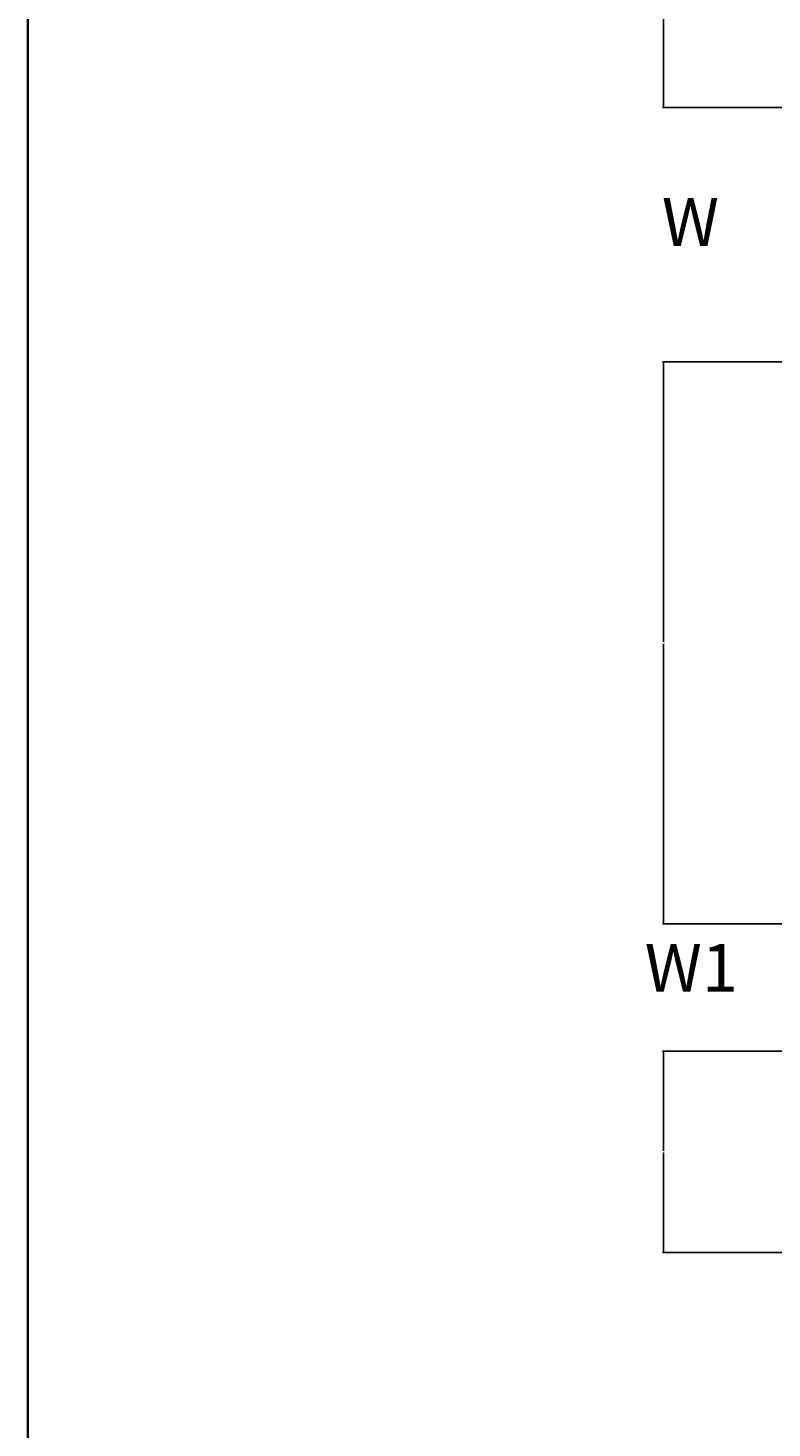
# Model space of a CAD drawing. Units: inches. Extents: x 2473 to 3664, y 1231 to 2079.
# Tile 2 of 8: x 2473 to 2614, y 1555 to 1819. Entities that reach past the tile are written whole.
import ezdxf

# ---------------------------------------------------------------- set-up
doc = ezdxf.new("R2010")
doc.units = ezdxf.units.IN
doc.linetypes.add('ACAD_ISO02W100', pattern=[15, 12, -3])
doc.layers.get('Defpoints').update_dxf_attribs({"linetype": 'ACAD_ISO02W100'})
for name, color, linetype, lineweight in [('A-ANNO-DIMS', 2, 'Continuous', 18), ('A-ANNO-IDEN', 7, 'Continuous', 18), ('A-ANNO-TTLB', 7, 'Continuous', 35)]:
    doc.layers.add(name, color=color, linetype=linetype, lineweight=lineweight)
doc.styles.get("Standard").update_dxf_attribs({"font": 'arial.ttf'})
doc.dimstyles.get("Standard").update_dxf_attribs({"dimtxt": 0.18, "dimasz": 0.18, "dimexe": 0.18, "dimexo": 0.0625, "dimgap": 0.09, "dimtad": 0, "dimtih": 1, "dimtoh": 1, "dimdec": 4, "dimzin": 0, "dimdsep": 46, "dimtxsty": 'Standard', "dimcen": 0.09, "dimadec": 0, "dimazin": 0, "dimtfac": 1, "dimtdec": 4, "dimtofl": 0, "dimtmove": 0, "dimatfit": 3, "dimfxl": 1, "dimtolj": 1, "dimtzin": 0, "dimarcsym": 0})

# ---------------------------------------------------------------- blocks, each defined once
blk = doc.blocks.new('*D57')
at = {"layer": 'A-ANNO-DIMS', "color": 0, "lineweight": -2, "transparency": 16777216}
for p, q in [((2617.6, 1626.06), (2593.03, 1626.06)), ((2593.21, 1625.88), (2593.21, 1607.24)), ((2593.21, 1588.24), (2593.21, 1606.87)), ((2617.6, 1588.06), (2593.03, 1588.06))]:
    blk.add_line(p, q, dxfattribs=at)
at = {"layer": 'A-ANNO-DIMS', "color": 0, "transparency": 16777216}
for points in [[(2593.18, 1625.88), (2593.24, 1625.88), (2593.21, 1626.06)], [(2593.18, 1588.24), (2593.24, 1588.24), (2593.21, 1588.06)]]:
    blk.add_solid(points, dxfattribs=at)
at = {"layer": 'Defpoints', "color": 0, "transparency": 16777216}
for p in [(2593.21, 1626.06), (2617.66, 1626.06), (2617.66, 1588.06)]:
    blk.add_point(p, dxfattribs=at)
at = {"layer": 'A-ANNO-DIMS', "color": 0, "transparency": 16777216, "insert": (2593.21, 1607.06), "char_height": 0.18, "attachment_point": 5}
blk.add_mtext('\\A1;38', dxfattribs=at)
blk = doc.blocks.new('*D58')
at = {"layer": 'A-ANNO-DIMS', "color": 0, "lineweight": -2, "transparency": 16777216}
for p, q in [((2617.6, 1756.06), (2593.03, 1756.06)), ((2593.21, 1755.88), (2593.21, 1703.24)), ((2593.21, 1650.24), (2593.21, 1702.87)), ((2617.6, 1650.06), (2593.03, 1650.06))]:
    blk.add_line(p, q, dxfattribs=at)
at = {"layer": 'A-ANNO-DIMS', "color": 0, "transparency": 16777216}
for points in [[(2593.18, 1755.88), (2593.24, 1755.88), (2593.21, 1756.06)], [(2593.18, 1650.24), (2593.24, 1650.24), (2593.21, 1650.06)]]:
    blk.add_solid(points, dxfattribs=at)
at = {"layer": 'Defpoints', "color": 0, "transparency": 16777216}
for p in [(2593.21, 1756.06), (2617.66, 1756.06), (2617.66, 1650.06)]:
    blk.add_point(p, dxfattribs=at)
at = {"layer": 'A-ANNO-DIMS', "color": 0, "transparency": 16777216, "insert": (2593.21, 1703.06), "char_height": 0.18, "attachment_point": 5}
blk.add_mtext('\\A1;106', dxfattribs=at)
blk = doc.blocks.new('*D59')
at = {"layer": 'A-ANNO-DIMS', "color": 0, "lineweight": -2, "transparency": 16777216}
for p, q in [((2617.597908, 1881.056109), (2593.030408, 1881.056109)), ((2593.210408, 1880.876109), (2593.210408, 1842.736109)), ((2593.210408, 1804.236109), (2593.210408, 1842.376109)), ((2617.597908, 1804.056109), (2593.030408, 1804.056109))]:
    blk.add_line(p, q, dxfattribs=at)
at = {"layer": 'A-ANNO-DIMS', "color": 0, "transparency": 16777216}
for points in [[(2593.180408, 1880.876109), (2593.240408, 1880.876109), (2593.210408, 1881.056109)], [(2593.180408, 1804.236109), (2593.240408, 1804.236109), (2593.210408, 1804.056109)]]:
    blk.add_solid(points, dxfattribs=at)
at = {"layer": 'Defpoints', "color": 0, "transparency": 16777216}
for p in [(2593.210408, 1881.056109), (2617.660408, 1881.056109), (2617.660408, 1804.056109)]:
    blk.add_point(p, dxfattribs=at)
at = {"layer": 'A-ANNO-DIMS', "color": 0, "transparency": 16777216, "insert": (2593.210408, 1842.556109), "char_height": 0.18, "attachment_point": 5}
blk.add_mtext('\\A1;77', dxfattribs=at)

msp = doc.modelspace()

# ---------------------------------------------------------------- linework, layer by layer
at = {"layer": 'A-ANNO-TTLB'}
msp.add_lwpolyline([(2473.2801, 2079.0861), (3663.7983, 2079.0861), (3663.7983, 1231.3065), (2473.2801, 1231.3065)], close=True, dxfattribs=at)

# ---------------------------------------------------------------- texts
at = {"layer": 'A-ANNO-IDEN'}
for s, p in [('            W', (2559.9112, 1777.957)), ('           W1', (2559.4262, 1637.2429))]:
    msp.add_text(s, height=9, dxfattribs=at).set_placement(p)

# ---------------------------------------------------------------- dimensions: what is measured, and where the dimension line sits
at = {"layer": 'A-ANNO-DIMS'}
for base, p1, p2, picture, middle in [((2593.2104, 1881.0561), (2617.6604, 1804.0561), (2617.6604, 1881.0561), '*D59', (2593.2104, 1842.5561)), ((2593.2104, 1756.0561), (2617.6604, 1650.0561), (2617.6604, 1756.0561), '*D58', (2593.2104, 1703.0561)), ((2593.2104, 1626.0561), (2617.6604, 1588.0561), (2617.6604, 1626.0561), '*D57', (2593.2104, 1607.0561))]:
    dim = msp.add_linear_dim(base=base, p1=p1, p2=p2, angle=90, dimstyle='Standard', override={"dimdec": 0, "dimlfac": 1, "dimrnd": 0, "dimzin": 0, "dimdsep": 46, "dimlunit": 2}, dxfattribs=at)
    dim.commit()
    dim.dimension.update_dxf_attribs({"geometry": picture, "text_midpoint": middle})

doc.saveas('drawing.dxf')
